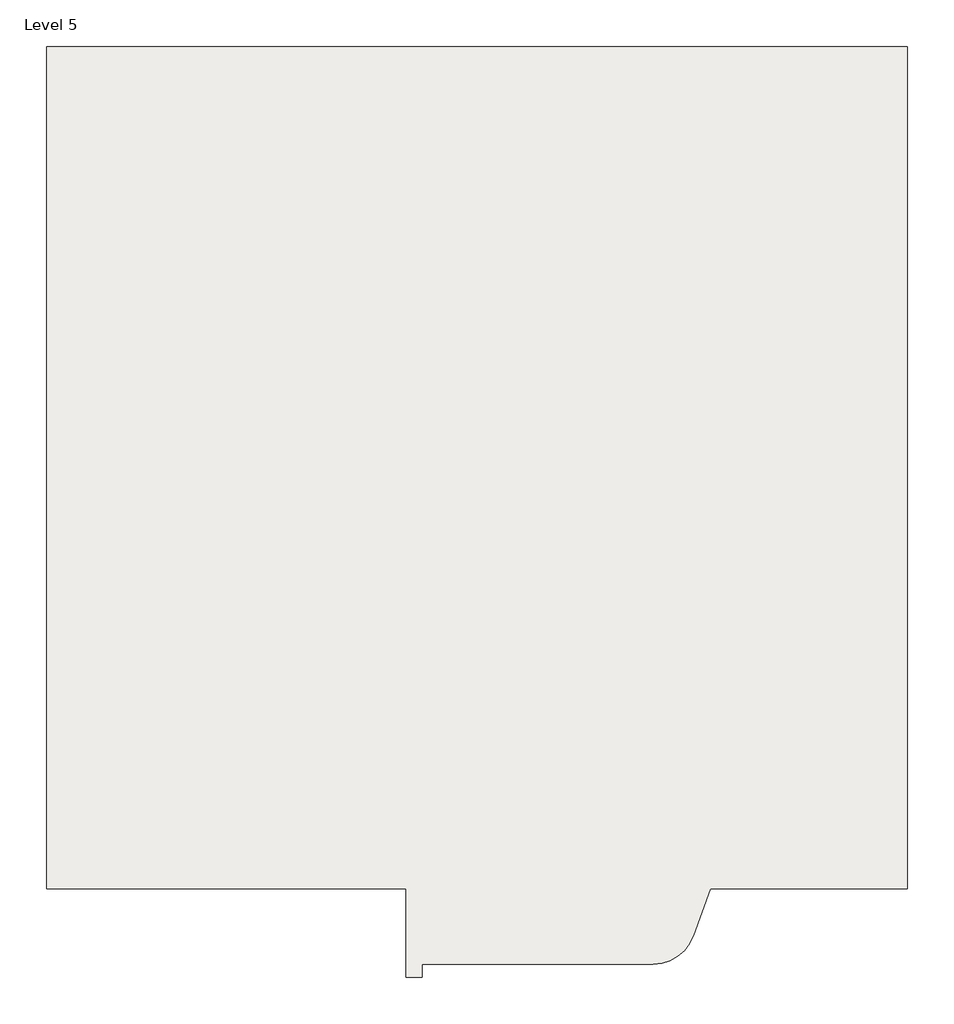
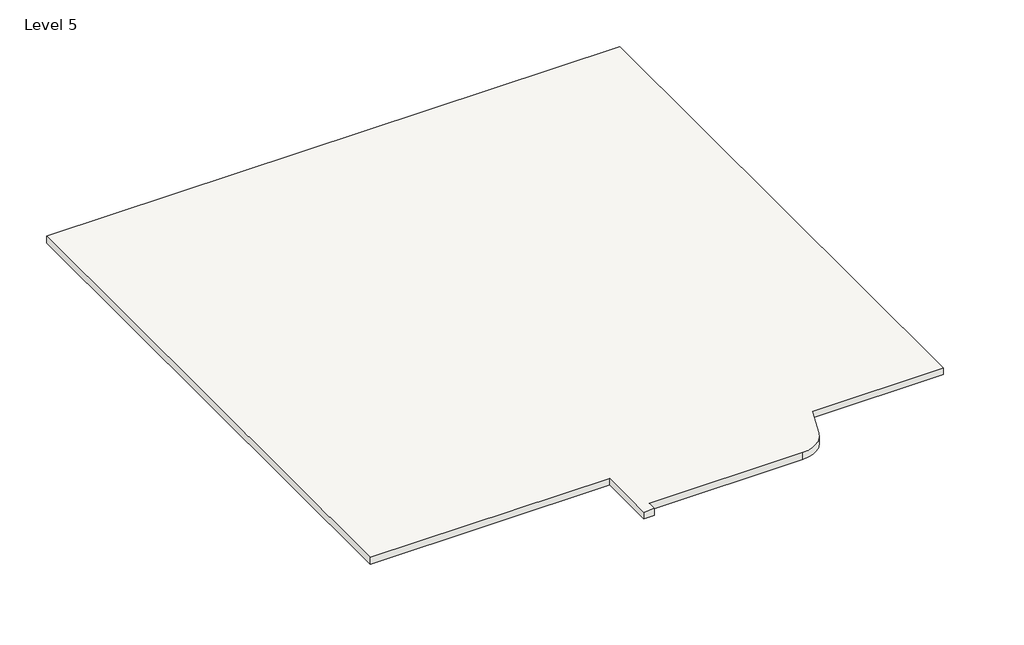
# One storey: 1 slab.
"""IFC4 building model written with IfcOpenShell, lengths in millimetres."""

from ifc_helpers import new_model, si_unit, point, frame, frame_2d, origin, place, context, project, spatial, polyline, circle_curve, trimmed, segment, composite_curve, outline, extrude, element, save

model = new_model("IFC4")

# Units and contexts
model_context = context("Model", 3, world=origin())
ifc_project = project(units=[si_unit("LENGTHUNIT", "METRE", prefix="MILLI")], contexts=[model_context])

# Site, building, storey
site = spatial("IfcSite", under=ifc_project)
building = spatial("IfcBuilding", under=site)
storey = spatial("IfcBuildingStorey", under=building, Name="Level 5", Elevation=9448.8)

# Slab
placement = place(None, origin())
element("IfcSlab", 1, ObjectType="6\" floor", at=placement, inside=storey, context=model_context, shape_type="SweptSolid", body=[
    extrude(outline(composite_curve([segment(polyline([(-2665.8678125, 13531.616018), (-2665.8678125, 1568.216018), (-5463.3133278, 1568.216018), (-5705.6066674, 902.5205386)]), True, "CONTINUOUS"), segment(trimmed(circle_curve(frame_2d((-6278.443289, 1111.016018)), 609.6), [point((-5705.6066674, 902.5205386))], [point((-6278.443289, 501.416018))], False, "CARTESIAN"), True, "CONTINUOUS"), segment(polyline([(-6278.443289, 501.416018), (-9561.9678125, 501.416018), (-9561.9678125, 310.916018), (-9790.5678125, 310.916018), (-9790.5678125, 1568.216018), (-14895.9678125, 1568.216018), (-14895.9678125, 13531.616018), (-2665.8678125, 13531.616018)]), True, "CONTINUOUS")], self_intersect=False)), frame((0.0, 0.0, 9296.4), z_axis=(0.0, 0.0, 1.0), x_axis=(1.0, 0.0, 0.0)), (0.0, 0.0, 1.0), 152.4),
])

save(model, "model.ifc")

# Revit data of these elements
# Type "6\" floor"
#   Assembly Code = "B1010"
#   Function = 0
#   Layers, outside or top first: 0' - 6" "Gypsum Wall Board" (function 1)
# Element 1 (IfcSlab, "6\" floor")
#   Height Offset From Level = 0' - 0"
#   Phase Created = New Construction
#   Materials on its faces: "Gypsum Wall Board"
# Materials
#   "Gypsum Wall Board": class "Generic", colour RGB 127 127 127, transparency 0, Description = "Gypsum Wall Board", Cost = 0
